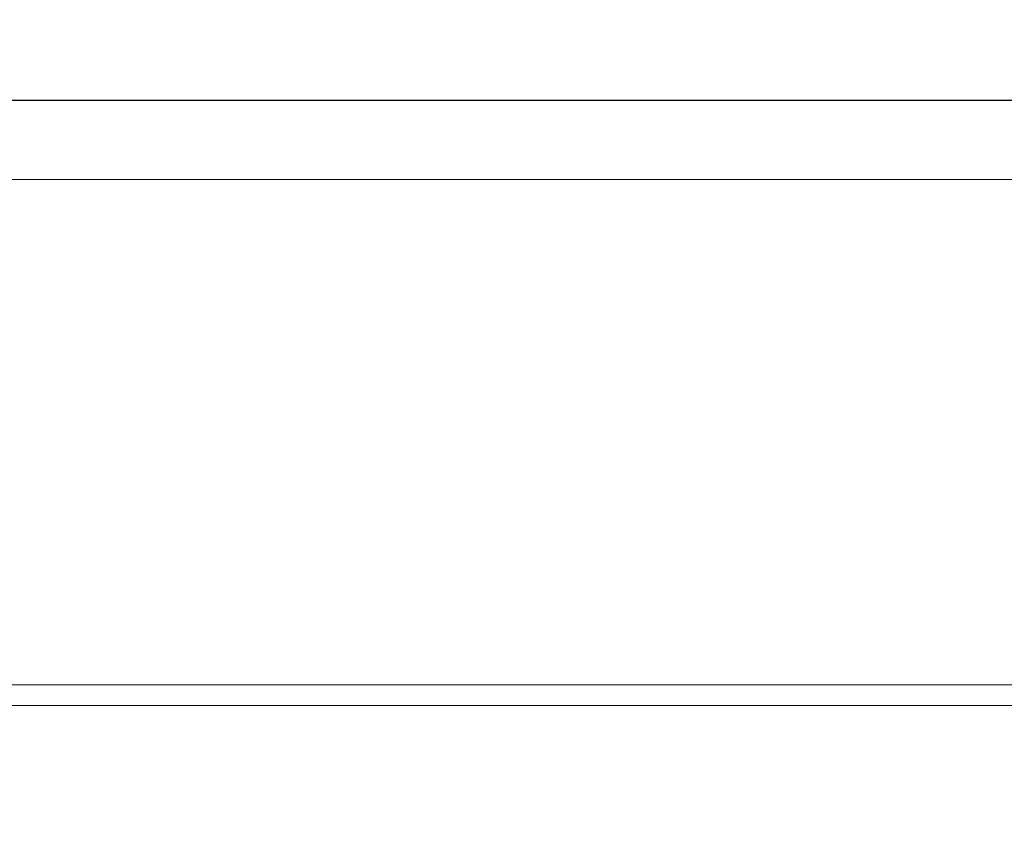
# Model space of a CAD drawing. Units: inches. Extents: x -1198 to -69, y -512 to 437.
# Tile 33 of 50: x -635.359 to -629.007, y 180.515 to 185.749. Entities that reach past the tile are written whole.
import ezdxf

# ---------------------------------------------------------------- set-up
doc = ezdxf.new("R2010")
doc.units = ezdxf.units.IN
doc.header["$MEASUREMENT"] = 0
for name, color, linetype, lineweight in [('0_Pen_No__7', 7, 'Continuous', 18), ('A-ANNO-DIMS', 2, 'Continuous', 18), ('A-EQPM', 60, 'Continuous', 18), ('A-FLOR-CASE', 7, 'Continuous', 25)]:
    doc.layers.add(name, color=color, linetype=linetype, lineweight=lineweight)
doc.styles.get("Standard").update_dxf_attribs({"font": 'arial.ttf'})
doc.dimstyles.get("Standard").update_dxf_attribs({"dimtxt": 6, "dimasz": 6, "dimexe": 0.18, "dimexo": 0.0625, "dimgap": 0.09, "dimtad": 0, "dimtih": 1, "dimtoh": 1, "dimdec": 0, "dimzin": 0, "dimdsep": 46, "dimlunit": 4, "dimtxsty": 'Standard', "dimblk": 'OBLIQUE', "dimcen": 0.09, "dimadec": 0, "dimazin": 0, "dimtfac": 1, "dimtdec": 0, "dimtofl": 0, "dimtmove": 0, "dimatfit": 3, "dimfxl": 1, "dimtolj": 1, "dimtzin": 0, "dimarcsym": 0})

# ---------------------------------------------------------------- blocks, each defined once
blk = doc.blocks.new('new block')
at = {"layer": '0_Pen_No__7'}
for p, q in [((-359, 99.11), (485.68, 99.11)), ((485.68, 95.73), (-359, 95.73))]:
    blk.add_line(p, q, dxfattribs=at)
blk.add_lwpolyline([(-354.49, 596.91), (481.18, 596.91, -0.414214), (485.68, 592.4), (485.68, 99.11), (486.24, 99.11), (486.24, 95.73), (485.68, 95.73), (485.68, 4.5, -0.414214), (481.18, 0), (-354.49, 0, -0.414214), (-359, 4.5), (-359, 95.73), (-359.56, 95.73), (-359.56, 99.11), (-359, 99.11), (-359, 592.4, -0.414214)], format="xyb", close=True, dxfattribs=at)
blk.add_lwpolyline([(-333.7, 12.95), (460.3, 12.95), (460.3, 570.44), (-333.7, 570.44)], close=True, dxfattribs=at)
blk = doc.blocks.new('COUNTER-L')
at = {"ltscale": 10}
blk.add_line((49.3491, 23.9997), (0.0001, 23.9997), dxfattribs=at)
blk = doc.blocks.new('_Oblique')
at = {"color": 0, "linetype": 'ByBlock', "lineweight": -2}
blk.add_line((-0.5, -0.5), (0.5, 0.5), dxfattribs=at)
blk = doc.blocks.new('*D56')
at = {"layer": 'A-ANNO-DIMS', "color": 0, "lineweight": -2, "ltscale": 10, "transparency": 16777216}
for p, q in [((-618.3394, 257.2277), (-603.8219, 257.2277)), ((-604.0019, 257.2277), (-604.0019, 212.422)), ((-604.0019, 161.2277), (-604.0019, 206.0333)), ((-618.3394, 161.2277), (-603.8219, 161.2277))]:
    blk.add_line(p, q, dxfattribs=at)
at = {"layer": 'DEFPOINTS', "color": 0, "ltscale": 10, "transparency": 16777216}
for p in [(-618.4019, 257.2277), (-604.0019, 257.2277), (-618.4019, 161.2277)]:
    blk.add_point(p, dxfattribs=at)
at = {"layer": 'A-ANNO-DIMS', "color": 0, "lineweight": -2, "ltscale": 10, "transparency": 16777216, "xscale": 6, "yscale": 6, "zscale": 6}
for p, rotation in [((-604.0019, 257.2277), 90), ((-604.0019, 161.2277), 270)]:
    blk.add_blockref('_Oblique', p, dxfattribs=dict(at, rotation=rotation))
at = {"layer": 'A-ANNO-DIMS', "color": 0, "ltscale": 10, "transparency": 16777216, "insert": (-604.0019, 209.2277), "char_height": 6, "attachment_point": 5}
blk.add_mtext('\\A1;COUNTER 96 TYP.', dxfattribs=at)

msp = doc.modelspace()

# ---------------------------------------------------------------- block references
at = {"layer": 'A-EQPM', "xscale": 0.0393700787401575, "yscale": 0.0393700787401575, "zscale": 0.0393700787401575, "rotation": 180}
msp.add_blockref('new block', (-638.3186, 185.2277), dxfattribs=at)
at = {"layer": 'A-FLOR-CASE'}
msp.add_blockref('COUNTER-L', (-667.751, 161.228), dxfattribs=at)

# ---------------------------------------------------------------- dimensions: what is measured, and where the dimension line sits
at = {"layer": 'A-ANNO-DIMS', "ltscale": 10}
dim = msp.add_linear_dim(base=(-604.0019, 257.2277), p1=(-618.4019, 161.2277), p2=(-618.4019, 257.2277), angle=90, text='COUNTER <> TYP.', dimstyle='Standard', override={"dimdec": 0, "dimlfac": 1, "dimrnd": 0, "dimzin": 0, "dimdsep": 46, "dimlunit": 2}, dxfattribs=at)
dim.commit()
dim.dimension.update_dxf_attribs({"geometry": '*D56', "text_midpoint": (-604.0019, 209.2277)})

doc.saveas('drawing.dxf')
